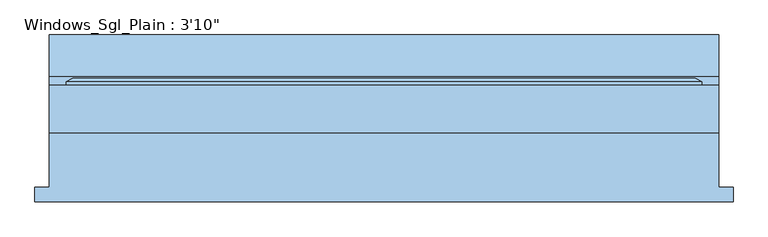
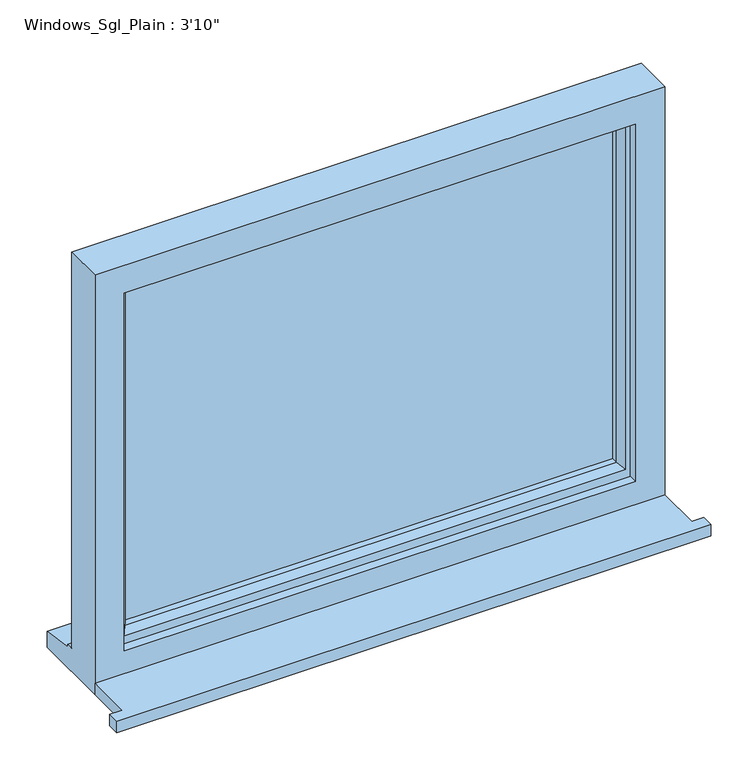
"""IFC4 building model written with IfcOpenShell, lengths in millimetres: window geometry."""

from ifc_helpers import new_model, si_unit, frame, origin, place, context, project, spatial, polyline, outline, extrude, faceted_brep, source, transform, mapped, element, save


def window_6a333e19(model_context):
    return source(origin(), model_context, "Body", "SolidModel", [
        extrude(outline(polyline([(-609.2, -130.8434322), (-609.2, -105.8434322), (-584.2, -105.8434322), (-584.2, -10.2434322), (584.2, -10.2434322), (584.2, -105.8434322), (609.2, -105.8434322), (609.2, -130.8434322), (-609.2, -130.8434322)])), frame((0.0, 0.0, 1200.0), z_axis=(0.0, 0.0, 1.0), x_axis=(1.0, 0.0, 0.0)), (0.0, 0.0, 1.0), 25.0),
        faceted_brep([(-584.2, -10.2434322, 1200.0), (584.2, -10.2434322, 1200.0), (584.2, -10.2434322, 2110.0), (-584.2, -10.2434322, 2110.0), (-524.2, -10.2434322, 2050.0), (524.2, -10.2434322, 2050.0), (524.2, -10.2434322, 1275.0), (-524.2, -10.2434322, 1275.0), (-584.2, 72.7565678, 2110.0), (-584.2, 72.7565678, 1251.0), (-584.2, 87.7565678, 1249.68767), (-584.2, 87.7565678, 1244.7449676), (-584.2, 160.2565678, 1233.8088847), (-584.2, 160.2565678, 1200.0), (584.2, 72.7565678, 2110.0), (584.2, 72.7565678, 1251.0), (-544.2, 72.7565678, 2070.0), (-544.2, 72.7565678, 1263.0), (544.2, 72.7565678, 1263.0), (544.2, 72.7565678, 2070.0), (-544.2, 7.7565678, 2070.0), (-544.2, 7.7565678, 1263.0), (544.2, 7.7565678, 2070.0), (544.2, 7.7565678, 1263.0), (-524.2, 7.7565678, 2050.0), (-524.2, 7.7565678, 1275.0), (524.2, 7.7565678, 1275.0), (524.2, 7.7565678, 2050.0), (584.2, 160.2565678, 1200.0), (584.2, 160.2565678, 1233.8088847), (584.2, 87.7565678, 1244.7449676), (584.2, 87.7565678, 1249.68767)], [[[0, 1, 2, 3], [4, 5, 6, 7]], [[0, 3, 8, 9, 10, 11, 12, 13]], [[9, 8, 14, 15], [16, 17, 18, 19]], [[17, 16, 20, 21]], [[20, 22, 23, 21], [24, 25, 26, 27]], [[24, 4, 7, 25]], [[3, 2, 14, 8]], [[16, 19, 22, 20]], [[5, 4, 24, 27]], [[15, 14, 2, 1, 28, 29, 30, 31]], [[19, 18, 23, 22]], [[5, 27, 26, 6]], [[28, 1, 0, 13]], [[29, 28, 13, 12]], [[30, 29, 12, 11]], [[31, 30, 11, 10]], [[15, 31, 10, 9]], [[21, 23, 18, 17]], [[7, 6, 26, 25]]]),
        extrude(outline(polyline([(514.2, 36.7565678), (-514.2, 36.7565678), (-514.2, 60.7565678), (514.2, 60.7565678), (514.2, 36.7565678)])), frame((0.0, 0.0, 1293.0), z_axis=(0.0, 0.0, 1.0), x_axis=(1.0, 0.0, 0.0)), (0.0, 0.0, 1.0), 747.0),
        faceted_brep([(-554.2, 72.7565678, 2080.0), (-554.2, 78.5300705, 2080.0), (-554.2, 78.5300705, 1253.0), (-554.2, 72.7565678, 1253.0), (-544.2, 7.7565678, 2070.0), (-544.2, 72.7565678, 2070.0), (-544.2, 72.7565678, 1263.0), (-544.2, 7.7565678, 1263.0), (-504.2, 22.2494677, 2030.0), (-514.3480377, 7.7565678, 2040.1480377), (-514.3480377, 7.7565678, 1292.8519623), (-504.2, 22.2494677, 1303.0), (-504.2, 36.7565678, 2030.0), (-504.2, 36.7565678, 1303.0), (-514.2, 60.7565678, 2040.0), (-514.2, 36.7565678, 2040.0), (-514.2, 36.7565678, 1293.0), (-514.2, 60.7565678, 1293.0), (-504.2, 78.5300705, 2030.0), (-504.2, 60.7565678, 2030.0), (-504.2, 60.7565678, 1303.0), (-504.2, 78.5300705, 1303.0), (-521.6457548, 84.3035732, 2047.4457548), (-521.6457548, 84.3035732, 1285.5542452), (-543.4153903, 84.3035732, 2069.2153903), (-543.4153903, 84.3035732, 1263.7846097), (554.2, 78.5300705, 1253.0), (554.2, 72.7565678, 1253.0), (544.2, 72.7565678, 1263.0), (544.2, 7.7565678, 1263.0), (514.3480377, 7.7565678, 1292.8519623), (504.2, 22.2494677, 1303.0), (504.2, 36.7565678, 1303.0), (514.2, 36.7565678, 1293.0), (514.2, 60.7565678, 1293.0), (504.2, 60.7565678, 1303.0), (504.2, 78.5300705, 1303.0), (521.6457548, 84.3035732, 1285.5542452), (543.4153903, 84.3035732, 1263.7846097), (554.2, 78.5300705, 2080.0), (554.2, 72.7565678, 2080.0), (544.2, 72.7565678, 2070.0), (544.2, 7.7565678, 2070.0), (514.3480377, 7.7565678, 2040.1480377), (504.2, 22.2494677, 2030.0), (504.2, 36.7565678, 2030.0), (514.2, 36.7565678, 2040.0), (514.2, 60.7565678, 2040.0), (504.2, 60.7565678, 2030.0), (504.2, 78.5300705, 2030.0), (521.6457548, 84.3035732, 2047.4457548), (543.4153903, 84.3035732, 2069.2153903)], [[[0, 1, 2, 3]], [[4, 5, 6, 7]], [[8, 9, 10, 11]], [[12, 8, 11, 13]], [[14, 15, 16, 17]], [[18, 19, 20, 21]], [[22, 18, 21, 23]], [[1, 24, 25, 2]], [[3, 2, 26, 27]], [[7, 6, 28, 29]], [[11, 10, 30, 31]], [[13, 11, 31, 32]], [[17, 16, 33, 34]], [[21, 20, 35, 36]], [[23, 21, 36, 37]], [[2, 25, 38, 26]], [[27, 26, 39, 40]], [[29, 28, 41, 42]], [[31, 30, 43, 44]], [[32, 31, 44, 45]], [[34, 33, 46, 47]], [[36, 35, 48, 49]], [[37, 36, 49, 50]], [[26, 38, 51, 39]], [[40, 39, 1, 0]], [[3, 27, 40, 0], [5, 41, 28, 6]], [[42, 41, 5, 4]], [[7, 29, 42, 4], [9, 43, 30, 10]], [[44, 43, 9, 8]], [[45, 44, 8, 12]], [[15, 46, 33, 16], [13, 32, 45, 12]], [[47, 46, 15, 14]], [[17, 34, 47, 14], [19, 48, 35, 20]], [[49, 48, 19, 18]], [[50, 49, 18, 22]], [[24, 51, 38, 25], [23, 37, 50, 22]], [[39, 51, 24, 1]]]),
    ])


if __name__ == "__main__":
    model = new_model("IFC4")
    model_context = context("Model", 3, world=origin())
    ifc_project = project(units=[si_unit("LENGTHUNIT", "METRE", prefix="MILLI")], contexts=[model_context])
    site = spatial("IfcSite", under=ifc_project)
    building = spatial("IfcBuilding", under=site)
    placement = place(None, origin())
    window_shape = window_6a333e19(model_context)
    element("IfcWindow", 1, ObjectType="Windows_Sgl_Plain : 3'10\"", at=placement, inside=building, context=model_context, shape_type="MappedRepresentation", body=[
        mapped(window_shape, transform((0.0, 0.0, 0.0), x_axis=(1.0, 0.0, 0.0), y_axis=(0.0, 1.0, 0.0), z_axis=(0.0, 0.0, 1.0))),
    ])
    save(model, "model.ifc")

# Revit data of these elements
# Type "Windows_Sgl_Plain : 3'10\""
#   Type Mark = "68"
#   Operation = "SinglePanel"
#   Construction Type Id = "SGL"
#   Manufacturer = "Revit"
#   Keynote = "L10"
#   Analytic Construction = "Large single-glazed windows"
#   Wrap Layers (Ext) from Ext = 0' - 4.03543"
#   Wrap Layers (Int) from Ext = 0' - 6.98819"
#   Window Board Projection = 0' - 0.98425"
#   Window Board Extension = 0' - 0.98425"
#   Visual Light Transmittance = 0.9
#   Solar Heat Gain Coefficient = 0.86
#   Rough Width = 3' - 10"
#   Rough Height = 2' - 11.82677"
#   Height = 2' - 11.82677"
#   Width = 3' - 10"
#   Heat Transfer Coefficient (U) = 5.5617 W/(m²·K)
#   Glazing Thickness = 0' - 0.94488"
#   FrameOffset - External = 0' - 1.9685"
#   Frame Depth = 0' - 2.55906"
#   Default Head Height = 6' - 11.07087"
#   Cill Depth = 0' - 3.44488"
#   Cavity Closer Width = 0' - 1.9685"
#   Cavity Closer Offset from Ext = 0' - 4.03543"
#   Cavity Closer Depth = 0' - 3.34646"
#   Vis - Cavity Closers = yes
#   Define Thermal Properties by = 1
#   Material Trim = Window Frame
#   Material Glass = Glass
#   Material Frame = Window Frame
#   Wall Closure = (empty or 0)
# Element 1 (IfcWindow, "Windows_Sgl_Plain : 3'10\"")
#   Materials on its faces: "Window Frame", "Glass"
# Materials
#   "Window Frame": colour RGB 249 249 249, transparency 0, Keynote = "L10", Cost = 0
#   "Glass": class "Glass", colour RGB 0 128 192, transparency 0.9, Description = "Soda Lime Glass", Cost = 0
